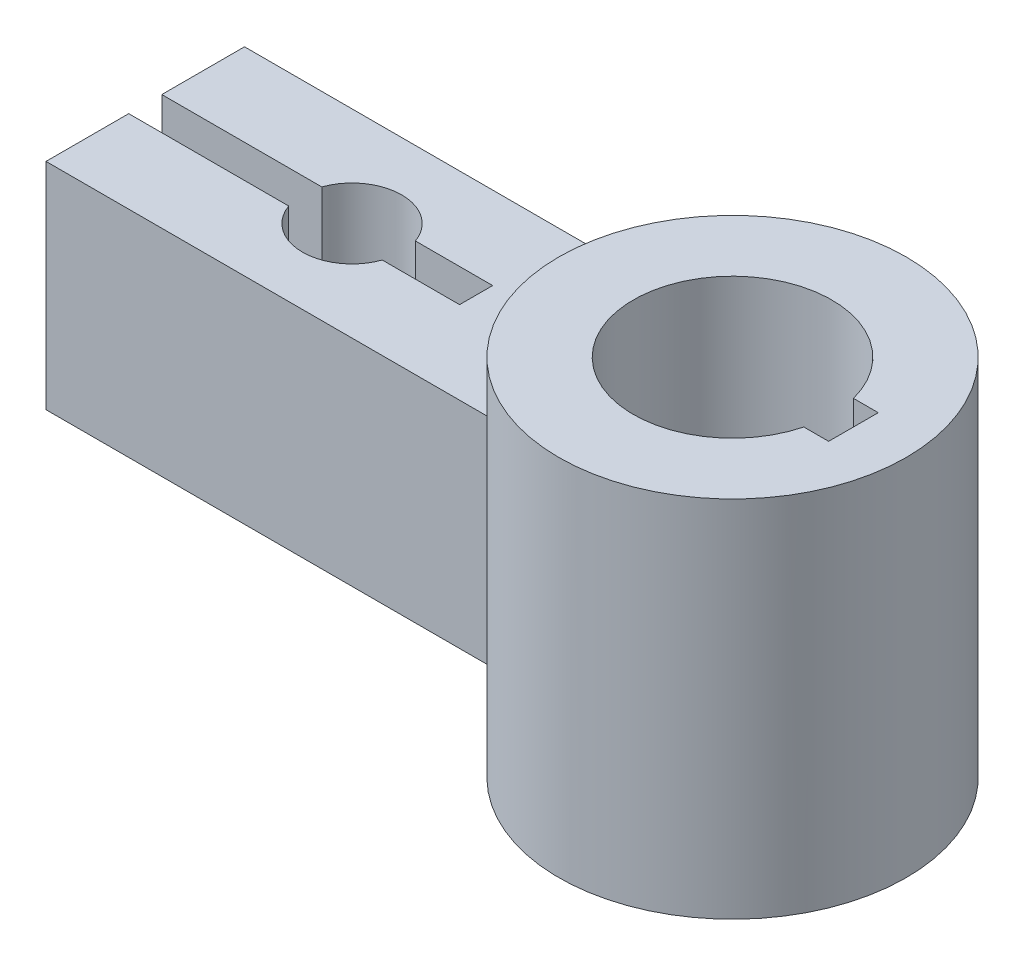
ISO-10303-21;
HEADER;
FILE_DESCRIPTION(('STEP AP214'),'2;1');
FILE_NAME('part.step','',(''),(''),'','','');
FILE_SCHEMA(('AUTOMOTIVE_DESIGN { 1 0 10303 214 1 1 1 1 }'));
ENDSEC;
DATA;
#1=APPLICATION_CONTEXT('core data for automotive mechanical design processes');
#2=APPLICATION_PROTOCOL_DEFINITION('international standard','automotive_design',2000,#1);
#3=PRODUCT_CONTEXT('',#1,'mechanical');
#4=PRODUCT('Part','Part','',(#3));
#5=PRODUCT_RELATED_PRODUCT_CATEGORY('part','',(#4));
#6=PRODUCT_DEFINITION_FORMATION('','',#4);
#7=PRODUCT_DEFINITION_CONTEXT('part definition',#1,'design');
#8=PRODUCT_DEFINITION('design','',#6,#7);
#9=PRODUCT_DEFINITION_SHAPE('','',#8);
#10=(LENGTH_UNIT() NAMED_UNIT(*) SI_UNIT(.MILLI.,.METRE.));
#11=(NAMED_UNIT(*) PLANE_ANGLE_UNIT() SI_UNIT($,.RADIAN.));
#12=(NAMED_UNIT(*) SI_UNIT($,.STERADIAN.) SOLID_ANGLE_UNIT());
#13=UNCERTAINTY_MEASURE_WITH_UNIT(LENGTH_MEASURE(1.E-05),#10,'distance_accuracy_value','');
#14=(GEOMETRIC_REPRESENTATION_CONTEXT(3) GLOBAL_UNCERTAINTY_ASSIGNED_CONTEXT((#13)) GLOBAL_UNIT_ASSIGNED_CONTEXT((#10,
#11,#12)) REPRESENTATION_CONTEXT('',''));
#15=CARTESIAN_POINT('',(0.,0.,0.));
#16=DIRECTION('',(0.,0.,1.));
#17=DIRECTION('',(1.,0.,0.));
#18=AXIS2_PLACEMENT_3D('',#15,#16,#17);
#19=CARTESIAN_POINT('',(0.,44.,0.));
#20=DIRECTION('',(0.,-1.,0.));
#21=DIRECTION('',(0.,0.,-1.));
#22=AXIS2_PLACEMENT_3D('',#19,#20,#21);
#23=CYLINDRICAL_SURFACE('',#22,21.);
#24=CARTESIAN_POINT('',(0.,44.,0.));
#25=DIRECTION('',(0.,1.,0.));
#26=DIRECTION('',(0.,0.,1.));
#27=AXIS2_PLACEMENT_3D('',#24,#25,#26);
#28=CIRCLE('',#27,21.);
#29=CARTESIAN_POINT('',(0.,44.,21.));
#30=VERTEX_POINT('',#29);
#31=EDGE_CURVE('E258',#30,#30,#28,.T.);
#32=ORIENTED_EDGE('',*,*,#31,.F.);
#33=EDGE_LOOP('',(#32));
#34=FACE_BOUND('',#33,.T.);
#35=DIRECTION('',(0.,-1.,0.));
#36=VECTOR('',#35,1.);
#37=CARTESIAN_POINT('',(0.,26.,-21.));
#38=LINE('',#37,#36);
#39=CARTESIAN_POINT('',(0.,26.,-21.));
#40=VERTEX_POINT('',#39);
#41=CARTESIAN_POINT('',(0.,0.,-21.));
#42=VERTEX_POINT('',#41);
#43=EDGE_CURVE('E62',#40,#42,#38,.T.);
#44=ORIENTED_EDGE('',*,*,#43,.F.);
#45=CARTESIAN_POINT('',(0.,26.,0.));
#46=DIRECTION('',(0.,1.,0.));
#47=DIRECTION('',(0.,0.,1.));
#48=AXIS2_PLACEMENT_3D('',#45,#46,#47);
#49=CIRCLE('',#48,21.);
#50=CARTESIAN_POINT('',(-20.7846096908265,26.,2.99999999999999));
#51=VERTEX_POINT('',#50);
#52=EDGE_CURVE('E57',#40,#51,#49,.T.);
#53=ORIENTED_EDGE('',*,*,#52,.T.);
#54=DIRECTION('',(0.,-1.,0.));
#55=VECTOR('',#54,1.);
#56=CARTESIAN_POINT('',(-20.7846096908265,26.,2.99999999999999));
#57=LINE('',#56,#55);
#58=CARTESIAN_POINT('',(-20.7846096908265,0.,2.99999999999999));
#59=VERTEX_POINT('',#58);
#60=EDGE_CURVE('E200',#51,#59,#57,.T.);
#61=ORIENTED_EDGE('',*,*,#60,.T.);
#62=CARTESIAN_POINT('',(0.,0.,0.));
#63=DIRECTION('',(0.,1.,0.));
#64=DIRECTION('',(0.,0.,1.));
#65=AXIS2_PLACEMENT_3D('',#62,#63,#64);
#66=CIRCLE('',#65,21.);
#67=EDGE_CURVE('E251',#59,#42,#66,.T.);
#68=ORIENTED_EDGE('',*,*,#67,.T.);
#69=EDGE_LOOP('',(#44,#53,#61,#68));
#70=FACE_BOUND('',#69,.T.);
#71=ADVANCED_FACE('F41',(#34,#70),#23,.T.);
#72=CARTESIAN_POINT('',(0.,44.,0.));
#73=DIRECTION('',(0.,-1.,0.));
#74=DIRECTION('',(0.,0.,-1.));
#75=AXIS2_PLACEMENT_3D('',#72,#73,#74);
#76=CYLINDRICAL_SURFACE('',#75,12.);
#77=CARTESIAN_POINT('',(0.,0.,0.));
#78=DIRECTION('',(0.,1.,0.));
#79=DIRECTION('',(0.,0.,1.));
#80=AXIS2_PLACEMENT_3D('',#77,#78,#79);
#81=CIRCLE('',#80,12.);
#82=CARTESIAN_POINT('',(11.6189500386223,0.,-3.));
#83=VERTEX_POINT('',#82);
#84=CARTESIAN_POINT('',(11.6189500386223,0.,3.));
#85=VERTEX_POINT('',#84);
#86=EDGE_CURVE('E248',#83,#85,#81,.T.);
#87=ORIENTED_EDGE('',*,*,#86,.F.);
#88=DIRECTION('',(0.,-1.,0.));
#89=VECTOR('',#88,1.);
#90=CARTESIAN_POINT('',(11.6189500386223,44.,-3.));
#91=LINE('',#90,#89);
#92=CARTESIAN_POINT('',(11.6189500386223,44.,-3.));
#93=VERTEX_POINT('',#92);
#94=EDGE_CURVE('E11',#93,#83,#91,.T.);
#95=ORIENTED_EDGE('',*,*,#94,.F.);
#96=CARTESIAN_POINT('',(0.,44.,0.));
#97=DIRECTION('',(0.,1.,0.));
#98=DIRECTION('',(0.,0.,1.));
#99=AXIS2_PLACEMENT_3D('',#96,#97,#98);
#100=CIRCLE('',#99,12.);
#101=CARTESIAN_POINT('',(11.6189500386223,44.,3.));
#102=VERTEX_POINT('',#101);
#103=EDGE_CURVE('E249',#93,#102,#100,.T.);
#104=ORIENTED_EDGE('',*,*,#103,.T.);
#105=DIRECTION('',(0.,-1.,0.));
#106=VECTOR('',#105,1.);
#107=CARTESIAN_POINT('',(11.6189500386223,44.,3.));
#108=LINE('',#107,#106);
#109=EDGE_CURVE('E262',#102,#85,#108,.T.);
#110=ORIENTED_EDGE('',*,*,#109,.T.);
#111=EDGE_LOOP('',(#87,#95,#104,#110));
#112=FACE_BOUND('',#111,.T.);
#113=ADVANCED_FACE('F43',(#112),#76,.F.);
#114=CARTESIAN_POINT('',(0.,44.,-3.));
#115=DIRECTION('',(0.,0.,-1.));
#116=DIRECTION('',(-1.,0.,0.));
#117=AXIS2_PLACEMENT_3D('',#114,#115,#116);
#118=PLANE('',#117);
#119=DIRECTION('',(1.,0.,0.));
#120=VECTOR('',#119,1.);
#121=CARTESIAN_POINT('',(0.,0.,-3.));
#122=LINE('',#121,#120);
#123=CARTESIAN_POINT('',(14.6189500386223,0.,-3.));
#124=VERTEX_POINT('',#123);
#125=EDGE_CURVE('E266',#83,#124,#122,.T.);
#126=ORIENTED_EDGE('',*,*,#125,.T.);
#127=DIRECTION('',(0.,-1.,0.));
#128=VECTOR('',#127,1.);
#129=CARTESIAN_POINT('',(14.6189500386223,44.,-3.));
#130=LINE('',#129,#128);
#131=CARTESIAN_POINT('',(14.6189500386223,44.,-3.));
#132=VERTEX_POINT('',#131);
#133=EDGE_CURVE('E47',#132,#124,#130,.T.);
#134=ORIENTED_EDGE('',*,*,#133,.F.);
#135=DIRECTION('',(1.,0.,0.));
#136=VECTOR('',#135,1.);
#137=CARTESIAN_POINT('',(0.,44.,-3.));
#138=LINE('',#137,#136);
#139=EDGE_CURVE('E254',#93,#132,#138,.T.);
#140=ORIENTED_EDGE('',*,*,#139,.F.);
#141=ORIENTED_EDGE('',*,*,#94,.T.);
#142=EDGE_LOOP('',(#126,#134,#140,#141));
#143=FACE_BOUND('',#142,.T.);
#144=ADVANCED_FACE('F297',(#143),#118,.F.);
#145=CARTESIAN_POINT('',(14.6189500386223,44.,0.));
#146=DIRECTION('',(1.,0.,0.));
#147=DIRECTION('',(0.,0.,-1.));
#148=AXIS2_PLACEMENT_3D('',#145,#146,#147);
#149=PLANE('',#148);
#150=DIRECTION('',(0.,0.,1.));
#151=VECTOR('',#150,1.);
#152=CARTESIAN_POINT('',(14.6189500386223,0.,0.));
#153=LINE('',#152,#151);
#154=CARTESIAN_POINT('',(14.6189500386223,0.,3.));
#155=VERTEX_POINT('',#154);
#156=EDGE_CURVE('E267',#124,#155,#153,.T.);
#157=ORIENTED_EDGE('',*,*,#156,.T.);
#158=DIRECTION('',(0.,-1.,0.));
#159=VECTOR('',#158,1.);
#160=CARTESIAN_POINT('',(14.6189500386223,44.,3.));
#161=LINE('',#160,#159);
#162=CARTESIAN_POINT('',(14.6189500386223,44.,3.));
#163=VERTEX_POINT('',#162);
#164=EDGE_CURVE('E273',#163,#155,#161,.T.);
#165=ORIENTED_EDGE('',*,*,#164,.F.);
#166=DIRECTION('',(0.,0.,1.));
#167=VECTOR('',#166,1.);
#168=CARTESIAN_POINT('',(14.6189500386223,44.,0.));
#169=LINE('',#168,#167);
#170=EDGE_CURVE('E257',#132,#163,#169,.T.);
#171=ORIENTED_EDGE('',*,*,#170,.F.);
#172=ORIENTED_EDGE('',*,*,#133,.T.);
#173=EDGE_LOOP('',(#157,#165,#171,#172));
#174=FACE_BOUND('',#173,.T.);
#175=ADVANCED_FACE('F284',(#174),#149,.F.);
#176=CARTESIAN_POINT('',(0.,44.,3.));
#177=DIRECTION('',(0.,0.,1.));
#178=DIRECTION('',(1.,0.,0.));
#179=AXIS2_PLACEMENT_3D('',#176,#177,#178);
#180=PLANE('',#179);
#181=DIRECTION('',(-1.,0.,0.));
#182=VECTOR('',#181,1.);
#183=CARTESIAN_POINT('',(0.,0.,3.));
#184=LINE('',#183,#182);
#185=EDGE_CURVE('E269',#155,#85,#184,.T.);
#186=ORIENTED_EDGE('',*,*,#185,.T.);
#187=ORIENTED_EDGE('',*,*,#109,.F.);
#188=DIRECTION('',(-1.,0.,0.));
#189=VECTOR('',#188,1.);
#190=CARTESIAN_POINT('',(0.,44.,3.));
#191=LINE('',#190,#189);
#192=EDGE_CURVE('E259',#163,#102,#191,.T.);
#193=ORIENTED_EDGE('',*,*,#192,.F.);
#194=ORIENTED_EDGE('',*,*,#164,.T.);
#195=EDGE_LOOP('',(#186,#187,#193,#194));
#196=FACE_BOUND('',#195,.T.);
#197=ADVANCED_FACE('F295',(#196),#180,.F.);
#198=CARTESIAN_POINT('',(0.,44.,0.));
#199=DIRECTION('',(0.,1.,0.));
#200=DIRECTION('',(0.,0.,1.));
#201=AXIS2_PLACEMENT_3D('',#198,#199,#200);
#202=PLANE('',#201);
#203=ORIENTED_EDGE('',*,*,#103,.F.);
#204=ORIENTED_EDGE('',*,*,#139,.T.);
#205=ORIENTED_EDGE('',*,*,#170,.T.);
#206=ORIENTED_EDGE('',*,*,#192,.T.);
#207=EDGE_LOOP('',(#203,#204,#205,#206));
#208=FACE_BOUND('',#207,.T.);
#209=ORIENTED_EDGE('',*,*,#31,.T.);
#210=EDGE_LOOP('',(#209));
#211=FACE_BOUND('',#210,.T.);
#212=ADVANCED_FACE('F296',(#208,#211),#202,.T.);
#213=CARTESIAN_POINT('',(0.,0.,0.));
#214=DIRECTION('',(0.,1.,0.));
#215=DIRECTION('',(0.,0.,1.));
#216=AXIS2_PLACEMENT_3D('',#213,#214,#215);
#217=PLANE('',#216);
#218=ORIENTED_EDGE('',*,*,#86,.T.);
#219=ORIENTED_EDGE('',*,*,#185,.F.);
#220=ORIENTED_EDGE('',*,*,#156,.F.);
#221=ORIENTED_EDGE('',*,*,#125,.F.);
#222=EDGE_LOOP('',(#218,#219,#220,#221));
#223=FACE_BOUND('',#222,.T.);
#224=ORIENTED_EDGE('',*,*,#67,.F.);
#225=DIRECTION('',(1.,0.,0.));
#226=VECTOR('',#225,1.);
#227=CARTESIAN_POINT('',(0.,0.,2.99999999999999));
#228=LINE('',#227,#226);
#229=CARTESIAN_POINT('',(-80.,0.,3.));
#230=VERTEX_POINT('',#229);
#231=EDGE_CURVE('E228',#230,#59,#228,.T.);
#232=ORIENTED_EDGE('',*,*,#231,.F.);
#233=DIRECTION('',(0.,0.,1.));
#234=VECTOR('',#233,1.);
#235=CARTESIAN_POINT('',(-80.,0.,0.));
#236=LINE('',#235,#234);
#237=CARTESIAN_POINT('',(-80.,0.,-6.99999999999999));
#238=VERTEX_POINT('',#237);
#239=EDGE_CURVE('E223',#238,#230,#236,.T.);
#240=ORIENTED_EDGE('',*,*,#239,.F.);
#241=DIRECTION('',(1.,0.,0.));
#242=VECTOR('',#241,1.);
#243=CARTESIAN_POINT('',(0.,0.,-6.99999999999997));
#244=LINE('',#243,#242);
#245=CARTESIAN_POINT('',(-60.6568542494924,0.,-6.99999999999999));
#246=VERTEX_POINT('',#245);
#247=EDGE_CURVE('E221',#238,#246,#244,.T.);
#248=ORIENTED_EDGE('',*,*,#247,.T.);
#249=CARTESIAN_POINT('',(-55.,0.,-8.99999999999998));
#250=DIRECTION('',(0.,1.,0.));
#251=DIRECTION('',(0.,0.,1.));
#252=AXIS2_PLACEMENT_3D('',#249,#250,#251);
#253=CIRCLE('',#252,6.);
#254=CARTESIAN_POINT('',(-49.3431457505076,0.,-6.99999999999998));
#255=VERTEX_POINT('',#254);
#256=EDGE_CURVE('E217',#246,#255,#253,.T.);
#257=ORIENTED_EDGE('',*,*,#256,.T.);
#258=DIRECTION('',(1.,0.,0.));
#259=VECTOR('',#258,1.);
#260=CARTESIAN_POINT('',(0.,0.,-6.99999999999998));
#261=LINE('',#260,#259);
#262=CARTESIAN_POINT('',(-40.,0.,-6.99999999999998));
#263=VERTEX_POINT('',#262);
#264=EDGE_CURVE('E213',#255,#263,#261,.T.);
#265=ORIENTED_EDGE('',*,*,#264,.T.);
#266=DIRECTION('',(0.,0.,-1.));
#267=VECTOR('',#266,1.);
#268=CARTESIAN_POINT('',(-40.,0.,0.));
#269=LINE('',#268,#267);
#270=CARTESIAN_POINT('',(-40.,0.,-11.));
#271=VERTEX_POINT('',#270);
#272=EDGE_CURVE('E215',#263,#271,#269,.T.);
#273=ORIENTED_EDGE('',*,*,#272,.T.);
#274=DIRECTION('',(-1.,0.,0.));
#275=VECTOR('',#274,1.);
#276=CARTESIAN_POINT('',(0.,0.,-11.));
#277=LINE('',#276,#275);
#278=CARTESIAN_POINT('',(-49.3431457505076,0.,-11.));
#279=VERTEX_POINT('',#278);
#280=EDGE_CURVE('E209',#271,#279,#277,.T.);
#281=ORIENTED_EDGE('',*,*,#280,.T.);
#282=CARTESIAN_POINT('',(-55.,0.,-8.99999999999998));
#283=DIRECTION('',(0.,1.,0.));
#284=DIRECTION('',(0.,0.,1.));
#285=AXIS2_PLACEMENT_3D('',#282,#283,#284);
#286=CIRCLE('',#285,5.99999999999999);
#287=CARTESIAN_POINT('',(-60.6568542494924,0.,-11.));
#288=VERTEX_POINT('',#287);
#289=EDGE_CURVE('E207',#279,#288,#286,.T.);
#290=ORIENTED_EDGE('',*,*,#289,.T.);
#291=DIRECTION('',(-1.,0.,0.));
#292=VECTOR('',#291,1.);
#293=CARTESIAN_POINT('',(0.,0.,-11.));
#294=LINE('',#293,#292);
#295=CARTESIAN_POINT('',(-80.,0.,-11.));
#296=VERTEX_POINT('',#295);
#297=EDGE_CURVE('E202',#288,#296,#294,.T.);
#298=ORIENTED_EDGE('',*,*,#297,.T.);
#299=DIRECTION('',(0.,0.,1.));
#300=VECTOR('',#299,1.);
#301=CARTESIAN_POINT('',(-80.,0.,0.));
#302=LINE('',#301,#300);
#303=CARTESIAN_POINT('',(-80.,0.,-21.));
#304=VERTEX_POINT('',#303);
#305=EDGE_CURVE('E201',#304,#296,#302,.T.);
#306=ORIENTED_EDGE('',*,*,#305,.F.);
#307=DIRECTION('',(-1.,0.,0.));
#308=VECTOR('',#307,1.);
#309=CARTESIAN_POINT('',(0.,0.,-21.));
#310=LINE('',#309,#308);
#311=EDGE_CURVE('E165',#42,#304,#310,.T.);
#312=ORIENTED_EDGE('',*,*,#311,.F.);
#313=EDGE_LOOP('',(#224,#232,#240,#248,#257,#265,#273,#281,#290,#298,#306,#312));
#314=FACE_BOUND('',#313,.T.);
#315=ADVANCED_FACE('F288',(#223,#314),#217,.F.);
#316=CARTESIAN_POINT('',(0.,26.,-21.));
#317=DIRECTION('',(0.,0.,1.));
#318=DIRECTION('',(1.,0.,0.));
#319=AXIS2_PLACEMENT_3D('',#316,#317,#318);
#320=PLANE('',#319);
#321=ORIENTED_EDGE('',*,*,#311,.T.);
#322=DIRECTION('',(0.,-1.,0.));
#323=VECTOR('',#322,1.);
#324=CARTESIAN_POINT('',(-80.,26.,-21.));
#325=LINE('',#324,#323);
#326=CARTESIAN_POINT('',(-80.,26.,-21.));
#327=VERTEX_POINT('',#326);
#328=EDGE_CURVE('E163',#327,#304,#325,.T.);
#329=ORIENTED_EDGE('',*,*,#328,.F.);
#330=DIRECTION('',(-1.,0.,0.));
#331=VECTOR('',#330,1.);
#332=CARTESIAN_POINT('',(0.,26.,-21.));
#333=LINE('',#332,#331);
#334=EDGE_CURVE('E153',#40,#327,#333,.T.);
#335=ORIENTED_EDGE('',*,*,#334,.F.);
#336=ORIENTED_EDGE('',*,*,#43,.T.);
#337=EDGE_LOOP('',(#321,#329,#335,#336));
#338=FACE_BOUND('',#337,.T.);
#339=ADVANCED_FACE('F162',(#338),#320,.F.);
#340=CARTESIAN_POINT('',(-80.,26.,0.));
#341=DIRECTION('',(1.,0.,0.));
#342=DIRECTION('',(0.,0.,-1.));
#343=AXIS2_PLACEMENT_3D('',#340,#341,#342);
#344=PLANE('',#343);
#345=ORIENTED_EDGE('',*,*,#305,.T.);
#346=DIRECTION('',(0.,-1.,0.));
#347=VECTOR('',#346,1.);
#348=CARTESIAN_POINT('',(-80.,26.,-11.));
#349=LINE('',#348,#347);
#350=CARTESIAN_POINT('',(-80.,26.,-11.));
#351=VERTEX_POINT('',#350);
#352=EDGE_CURVE('E166',#351,#296,#349,.T.);
#353=ORIENTED_EDGE('',*,*,#352,.F.);
#354=DIRECTION('',(0.,0.,1.));
#355=VECTOR('',#354,1.);
#356=CARTESIAN_POINT('',(-80.,26.,0.));
#357=LINE('',#356,#355);
#358=EDGE_CURVE('E156',#327,#351,#357,.T.);
#359=ORIENTED_EDGE('',*,*,#358,.F.);
#360=ORIENTED_EDGE('',*,*,#328,.T.);
#361=EDGE_LOOP('',(#345,#353,#359,#360));
#362=FACE_BOUND('',#361,.T.);
#363=ADVANCED_FACE('F167',(#362),#344,.F.);
#364=CARTESIAN_POINT('',(0.,26.,-11.));
#365=DIRECTION('',(0.,0.,1.));
#366=DIRECTION('',(1.,0.,0.));
#367=AXIS2_PLACEMENT_3D('',#364,#365,#366);
#368=PLANE('',#367);
#369=ORIENTED_EDGE('',*,*,#297,.F.);
#370=DIRECTION('',(0.,-1.,0.));
#371=VECTOR('',#370,1.);
#372=CARTESIAN_POINT('',(-60.6568542494924,26.,-11.));
#373=LINE('',#372,#371);
#374=CARTESIAN_POINT('',(-60.6568542494924,26.,-11.));
#375=VERTEX_POINT('',#374);
#376=EDGE_CURVE('E244',#375,#288,#373,.T.);
#377=ORIENTED_EDGE('',*,*,#376,.F.);
#378=DIRECTION('',(-1.,0.,0.));
#379=VECTOR('',#378,1.);
#380=CARTESIAN_POINT('',(0.,26.,-11.));
#381=LINE('',#380,#379);
#382=EDGE_CURVE('E175',#375,#351,#381,.T.);
#383=ORIENTED_EDGE('',*,*,#382,.T.);
#384=ORIENTED_EDGE('',*,*,#352,.T.);
#385=EDGE_LOOP('',(#369,#377,#383,#384));
#386=FACE_BOUND('',#385,.T.);
#387=ADVANCED_FACE('F365',(#386),#368,.T.);
#388=CARTESIAN_POINT('',(-55.,26.,-8.99999999999998));
#389=DIRECTION('',(0.,-1.,0.));
#390=DIRECTION('',(0.,0.,-1.));
#391=AXIS2_PLACEMENT_3D('',#388,#389,#390);
#392=CYLINDRICAL_SURFACE('',#391,5.99999999999999);
#393=ORIENTED_EDGE('',*,*,#289,.F.);
#394=DIRECTION('',(0.,-1.,0.));
#395=VECTOR('',#394,1.);
#396=CARTESIAN_POINT('',(-49.3431457505076,26.,-11.));
#397=LINE('',#396,#395);
#398=CARTESIAN_POINT('',(-49.3431457505076,26.,-11.));
#399=VERTEX_POINT('',#398);
#400=EDGE_CURVE('E243',#399,#279,#397,.T.);
#401=ORIENTED_EDGE('',*,*,#400,.F.);
#402=CARTESIAN_POINT('',(-55.,26.,-8.99999999999998));
#403=DIRECTION('',(0.,1.,0.));
#404=DIRECTION('',(0.,0.,1.));
#405=AXIS2_PLACEMENT_3D('',#402,#403,#404);
#406=CIRCLE('',#405,5.99999999999999);
#407=EDGE_CURVE('E172',#399,#375,#406,.T.);
#408=ORIENTED_EDGE('',*,*,#407,.T.);
#409=ORIENTED_EDGE('',*,*,#376,.T.);
#410=EDGE_LOOP('',(#393,#401,#408,#409));
#411=FACE_BOUND('',#410,.T.);
#412=ADVANCED_FACE('F369',(#411),#392,.F.);
#413=CARTESIAN_POINT('',(0.,26.,-11.));
#414=DIRECTION('',(0.,0.,1.));
#415=DIRECTION('',(1.,0.,0.));
#416=AXIS2_PLACEMENT_3D('',#413,#414,#415);
#417=PLANE('',#416);
#418=ORIENTED_EDGE('',*,*,#280,.F.);
#419=DIRECTION('',(0.,-1.,0.));
#420=VECTOR('',#419,1.);
#421=CARTESIAN_POINT('',(-40.,26.,-11.));
#422=LINE('',#421,#420);
#423=CARTESIAN_POINT('',(-40.,26.,-11.));
#424=VERTEX_POINT('',#423);
#425=EDGE_CURVE('E241',#424,#271,#422,.T.);
#426=ORIENTED_EDGE('',*,*,#425,.F.);
#427=DIRECTION('',(-1.,0.,0.));
#428=VECTOR('',#427,1.);
#429=CARTESIAN_POINT('',(0.,26.,-11.));
#430=LINE('',#429,#428);
#431=EDGE_CURVE('E179',#424,#399,#430,.T.);
#432=ORIENTED_EDGE('',*,*,#431,.T.);
#433=ORIENTED_EDGE('',*,*,#400,.T.);
#434=EDGE_LOOP('',(#418,#426,#432,#433));
#435=FACE_BOUND('',#434,.T.);
#436=ADVANCED_FACE('F378',(#435),#417,.T.);
#437=CARTESIAN_POINT('',(-40.,26.,0.));
#438=DIRECTION('',(-1.,0.,0.));
#439=DIRECTION('',(0.,0.,1.));
#440=AXIS2_PLACEMENT_3D('',#437,#438,#439);
#441=PLANE('',#440);
#442=ORIENTED_EDGE('',*,*,#272,.F.);
#443=DIRECTION('',(0.,-1.,0.));
#444=VECTOR('',#443,1.);
#445=CARTESIAN_POINT('',(-40.,26.,-6.99999999999998));
#446=LINE('',#445,#444);
#447=CARTESIAN_POINT('',(-40.,26.,-6.99999999999998));
#448=VERTEX_POINT('',#447);
#449=EDGE_CURVE('E237',#448,#263,#446,.T.);
#450=ORIENTED_EDGE('',*,*,#449,.F.);
#451=DIRECTION('',(0.,0.,-1.));
#452=VECTOR('',#451,1.);
#453=CARTESIAN_POINT('',(-40.,26.,0.));
#454=LINE('',#453,#452);
#455=EDGE_CURVE('E182',#448,#424,#454,.T.);
#456=ORIENTED_EDGE('',*,*,#455,.T.);
#457=ORIENTED_EDGE('',*,*,#425,.T.);
#458=EDGE_LOOP('',(#442,#450,#456,#457));
#459=FACE_BOUND('',#458,.T.);
#460=ADVANCED_FACE('F389',(#459),#441,.T.);
#461=CARTESIAN_POINT('',(0.,26.,-6.99999999999998));
#462=DIRECTION('',(0.,0.,-1.));
#463=DIRECTION('',(-1.,0.,0.));
#464=AXIS2_PLACEMENT_3D('',#461,#462,#463);
#465=PLANE('',#464);
#466=ORIENTED_EDGE('',*,*,#264,.F.);
#467=DIRECTION('',(0.,-1.,0.));
#468=VECTOR('',#467,1.);
#469=CARTESIAN_POINT('',(-49.3431457505076,26.,-6.99999999999998));
#470=LINE('',#469,#468);
#471=CARTESIAN_POINT('',(-49.3431457505076,26.,-6.99999999999998));
#472=VERTEX_POINT('',#471);
#473=EDGE_CURVE('E240',#472,#255,#470,.T.);
#474=ORIENTED_EDGE('',*,*,#473,.F.);
#475=DIRECTION('',(1.,0.,0.));
#476=VECTOR('',#475,1.);
#477=CARTESIAN_POINT('',(0.,26.,-6.99999999999998));
#478=LINE('',#477,#476);
#479=EDGE_CURVE('E187',#472,#448,#478,.T.);
#480=ORIENTED_EDGE('',*,*,#479,.T.);
#481=ORIENTED_EDGE('',*,*,#449,.T.);
#482=EDGE_LOOP('',(#466,#474,#480,#481));
#483=FACE_BOUND('',#482,.T.);
#484=ADVANCED_FACE('F400',(#483),#465,.T.);
#485=CARTESIAN_POINT('',(-55.,26.,-8.99999999999998));
#486=DIRECTION('',(0.,-1.,0.));
#487=DIRECTION('',(0.,0.,-1.));
#488=AXIS2_PLACEMENT_3D('',#485,#486,#487);
#489=CYLINDRICAL_SURFACE('',#488,6.);
#490=ORIENTED_EDGE('',*,*,#256,.F.);
#491=DIRECTION('',(0.,-1.,0.));
#492=VECTOR('',#491,1.);
#493=CARTESIAN_POINT('',(-60.6568542494924,26.,-6.99999999999999));
#494=LINE('',#493,#492);
#495=CARTESIAN_POINT('',(-60.6568542494924,26.,-6.99999999999999));
#496=VERTEX_POINT('',#495);
#497=EDGE_CURVE('E232',#496,#246,#494,.T.);
#498=ORIENTED_EDGE('',*,*,#497,.F.);
#499=CARTESIAN_POINT('',(-55.,26.,-8.99999999999998));
#500=DIRECTION('',(0.,1.,0.));
#501=DIRECTION('',(0.,0.,1.));
#502=AXIS2_PLACEMENT_3D('',#499,#500,#501);
#503=CIRCLE('',#502,6.);
#504=EDGE_CURVE('E186',#496,#472,#503,.T.);
#505=ORIENTED_EDGE('',*,*,#504,.T.);
#506=ORIENTED_EDGE('',*,*,#473,.T.);
#507=EDGE_LOOP('',(#490,#498,#505,#506));
#508=FACE_BOUND('',#507,.T.);
#509=ADVANCED_FACE('F407',(#508),#489,.F.);
#510=CARTESIAN_POINT('',(0.,26.,-6.99999999999997));
#511=DIRECTION('',(0.,0.,-1.));
#512=DIRECTION('',(-1.,0.,0.));
#513=AXIS2_PLACEMENT_3D('',#510,#511,#512);
#514=PLANE('',#513);
#515=ORIENTED_EDGE('',*,*,#247,.F.);
#516=DIRECTION('',(0.,-1.,0.));
#517=VECTOR('',#516,1.);
#518=CARTESIAN_POINT('',(-80.,26.,-6.99999999999999));
#519=LINE('',#518,#517);
#520=CARTESIAN_POINT('',(-80.,26.,-6.99999999999999));
#521=VERTEX_POINT('',#520);
#522=EDGE_CURVE('E231',#521,#238,#519,.T.);
#523=ORIENTED_EDGE('',*,*,#522,.F.);
#524=DIRECTION('',(1.,0.,0.));
#525=VECTOR('',#524,1.);
#526=CARTESIAN_POINT('',(0.,26.,-6.99999999999997));
#527=LINE('',#526,#525);
#528=EDGE_CURVE('E195',#521,#496,#527,.T.);
#529=ORIENTED_EDGE('',*,*,#528,.T.);
#530=ORIENTED_EDGE('',*,*,#497,.T.);
#531=EDGE_LOOP('',(#515,#523,#529,#530));
#532=FACE_BOUND('',#531,.T.);
#533=ADVANCED_FACE('F411',(#532),#514,.T.);
#534=CARTESIAN_POINT('',(-80.,26.,0.));
#535=DIRECTION('',(1.,0.,0.));
#536=DIRECTION('',(0.,0.,-1.));
#537=AXIS2_PLACEMENT_3D('',#534,#535,#536);
#538=PLANE('',#537);
#539=ORIENTED_EDGE('',*,*,#239,.T.);
#540=DIRECTION('',(0.,-1.,0.));
#541=VECTOR('',#540,1.);
#542=CARTESIAN_POINT('',(-80.,26.,3.));
#543=LINE('',#542,#541);
#544=CARTESIAN_POINT('',(-80.,26.,3.));
#545=VERTEX_POINT('',#544);
#546=EDGE_CURVE('E229',#545,#230,#543,.T.);
#547=ORIENTED_EDGE('',*,*,#546,.F.);
#548=DIRECTION('',(0.,0.,1.));
#549=VECTOR('',#548,1.);
#550=CARTESIAN_POINT('',(-80.,26.,0.));
#551=LINE('',#550,#549);
#552=EDGE_CURVE('E193',#521,#545,#551,.T.);
#553=ORIENTED_EDGE('',*,*,#552,.F.);
#554=ORIENTED_EDGE('',*,*,#522,.T.);
#555=EDGE_LOOP('',(#539,#547,#553,#554));
#556=FACE_BOUND('',#555,.T.);
#557=ADVANCED_FACE('F425',(#556),#538,.F.);
#558=CARTESIAN_POINT('',(0.,26.,2.99999999999999));
#559=DIRECTION('',(0.,0.,-1.));
#560=DIRECTION('',(-1.,0.,0.));
#561=AXIS2_PLACEMENT_3D('',#558,#559,#560);
#562=PLANE('',#561);
#563=ORIENTED_EDGE('',*,*,#231,.T.);
#564=ORIENTED_EDGE('',*,*,#60,.F.);
#565=DIRECTION('',(1.,0.,0.));
#566=VECTOR('',#565,1.);
#567=CARTESIAN_POINT('',(0.,26.,2.99999999999999));
#568=LINE('',#567,#566);
#569=EDGE_CURVE('E199',#545,#51,#568,.T.);
#570=ORIENTED_EDGE('',*,*,#569,.F.);
#571=ORIENTED_EDGE('',*,*,#546,.T.);
#572=EDGE_LOOP('',(#563,#564,#570,#571));
#573=FACE_BOUND('',#572,.T.);
#574=ADVANCED_FACE('F433',(#573),#562,.F.);
#575=CARTESIAN_POINT('',(0.,26.,0.));
#576=DIRECTION('',(0.,1.,0.));
#577=DIRECTION('',(0.,0.,1.));
#578=AXIS2_PLACEMENT_3D('',#575,#576,#577);
#579=PLANE('',#578);
#580=ORIENTED_EDGE('',*,*,#52,.F.);
#581=ORIENTED_EDGE('',*,*,#334,.T.);
#582=ORIENTED_EDGE('',*,*,#358,.T.);
#583=ORIENTED_EDGE('',*,*,#382,.F.);
#584=ORIENTED_EDGE('',*,*,#407,.F.);
#585=ORIENTED_EDGE('',*,*,#431,.F.);
#586=ORIENTED_EDGE('',*,*,#455,.F.);
#587=ORIENTED_EDGE('',*,*,#479,.F.);
#588=ORIENTED_EDGE('',*,*,#504,.F.);
#589=ORIENTED_EDGE('',*,*,#528,.F.);
#590=ORIENTED_EDGE('',*,*,#552,.T.);
#591=ORIENTED_EDGE('',*,*,#569,.T.);
#592=EDGE_LOOP('',(#580,#581,#582,#583,#584,#585,#586,#587,#588,#589,#590,#591));
#593=FACE_BOUND('',#592,.T.);
#594=ADVANCED_FACE('F152',(#593),#579,.T.);
#595=CLOSED_SHELL('',(#71,#113,#144,#175,#197,#212,#315,#339,#363,#387,#412,#436,#460,#484,#509,
#533,#557,#574,#594));
#596=MANIFOLD_SOLID_BREP('B2',#595);
#597=ADVANCED_BREP_SHAPE_REPRESENTATION('',(#18,#596),#14);
#598=SHAPE_DEFINITION_REPRESENTATION(#9,#597);
ENDSEC;
END-ISO-10303-21;
